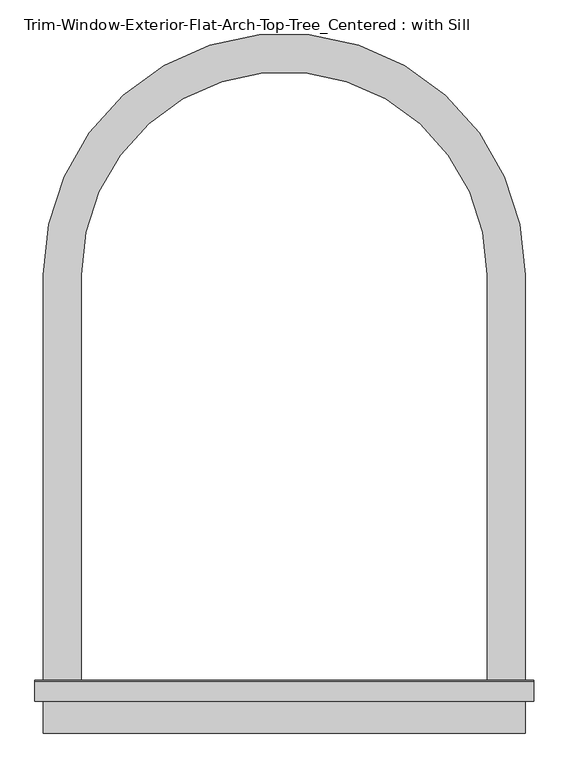
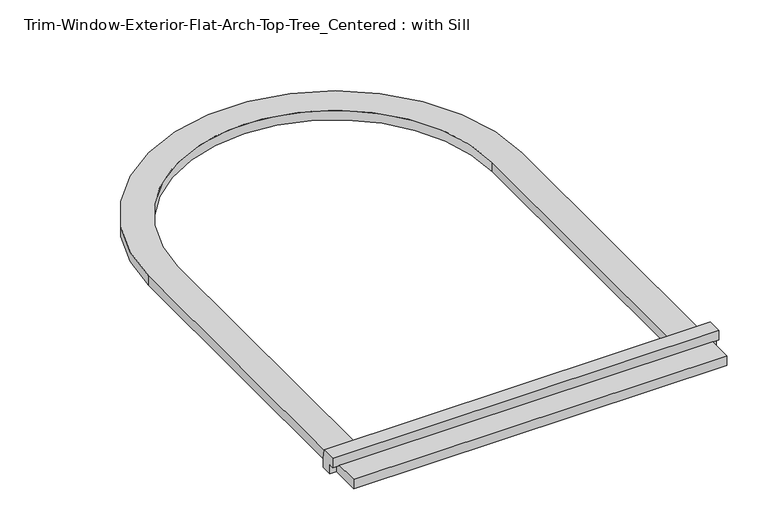
"""IFC4 building model written with IfcOpenShell, lengths in millimetres: proxy geometry, Trim-Window-Exterior-Flat-Arch-Top-Tree_Centered : with Sill."""

from ifc_helpers import new_model, si_unit, point, frame, frame_2d, origin, origin_with_axes, place, context, project, spatial, polyline, circle_curve, trimmed, segment, composite_curve, outline, extrude, source, transform, mapped, element, save


def trim_window_exterior_flat_arch_top_tree_centered_with_sill_b3d54518(model_context):
    return source(origin(), model_context, "Body", "SweptSolid", [
        extrude(outline(polyline([(361.95, -936.5823709), (361.95, -993.7323709), (-361.95, -993.7323709), (-361.95, -936.5823709), (361.95, -936.5823709)])), origin_with_axes(), (0.0, 0.0, 1.0), 19.05),
        extrude(outline(polyline([(-946.15, 38.1), (-916.8580645, 38.1), (-914.4, 19.05), (-914.4, 0.0), (-936.5823709, 0.0), (-936.5823709, 19.05), (-946.15, 19.05), (-946.15, 38.1)])), frame((-374.65, 0.0, 0.0), z_axis=(1.0, 0.0, 0.0), x_axis=(0.0, 1.0, 0.0)), (0.0, 0.0, 1.0), 749.3),
        extrude(outline(composite_curve([segment(trimmed(circle_curve(frame_2d((0.0, -304.8)), 361.95), [point((-361.95, -304.8))], [point((361.95, -304.8))], False, "CARTESIAN"), True, "CONTINUOUS"), segment(polyline([(361.95, -304.8), (361.95, -914.4), (304.8, -914.4), (304.8, -304.8)]), True, "CONTINUOUS"), segment(trimmed(circle_curve(frame_2d((0.0, -304.8)), 304.8), [point((304.8, -304.8))], [point((-304.8, -304.8))], True, "CARTESIAN"), True, "CONTINUOUS"), segment(polyline([(-304.8, -304.8), (-304.8, -914.4), (-361.95, -914.4), (-361.95, -304.8)]), True, "CONTINUOUS")], self_intersect=False)), origin_with_axes(), (0.0, 0.0, 1.0), 19.05),
    ])


if __name__ == "__main__":
    model = new_model("IFC4")
    model_context = context("Model", 3, world=origin())
    ifc_project = project(units=[si_unit("LENGTHUNIT", "METRE", prefix="MILLI")], contexts=[model_context])
    site = spatial("IfcSite", under=ifc_project)
    building = spatial("IfcBuilding", under=site)
    placement = place(None, origin())
    trim_window_exterior_flat_arch_top_tree_centered_with_sill_shape = trim_window_exterior_flat_arch_top_tree_centered_with_sill_b3d54518(model_context)
    element("IfcBuildingElementProxy", 1, Name="Trim-Window-Exterior-Flat-Arch-Top-Tree_Centered : with Sill", ObjectType="Trim-Window-Exterior-Flat-Arch-Top-Tree_Centered : with Sill", at=placement, inside=building, context=model_context, shape_type="MappedRepresentation", body=[
        mapped(trim_window_exterior_flat_arch_top_tree_centered_with_sill_shape, transform((0.0, 0.0, 0.0), x_axis=(1.0, 0.0, 0.0), y_axis=(0.0, 1.0, 0.0), z_axis=(0.0, 0.0, 1.0))),
    ])
    save(model, "model.ifc")

# Revit data of these elements
# Type "Trim-Window-Exterior-Flat-Arch-Top-Tree_Centered : with Sill"
#   Trim Width = 0' - 2 1/4"
#   Trim Thickness_Picture Frame = 0' - 1 1/4"
#   Trim Thickness_with Sill = 0' - 0 3/4"
#   Sill Thickness = 0' - 1 1/4"
#   Opening Width [instance default] = 2' - 0"
#   Opening Height [instance default] = 3' - 0"
#   Default Elevation = 4' - 0"
#   Sill = yes
#   Picture Frame = no
#   Trim Material [instance default] = none
# Element 1 (IfcBuildingElementProxy, "Trim-Window-Exterior-Flat-Arch-Top-Tree_Centered : with Sill")
#   Trim Material = Clad - White
#   Materials on its faces: "Clad - White"
# Materials
#   "Clad - White": class "Wood", colour RGB 242 242 238, transparency 0, Cost = 0
